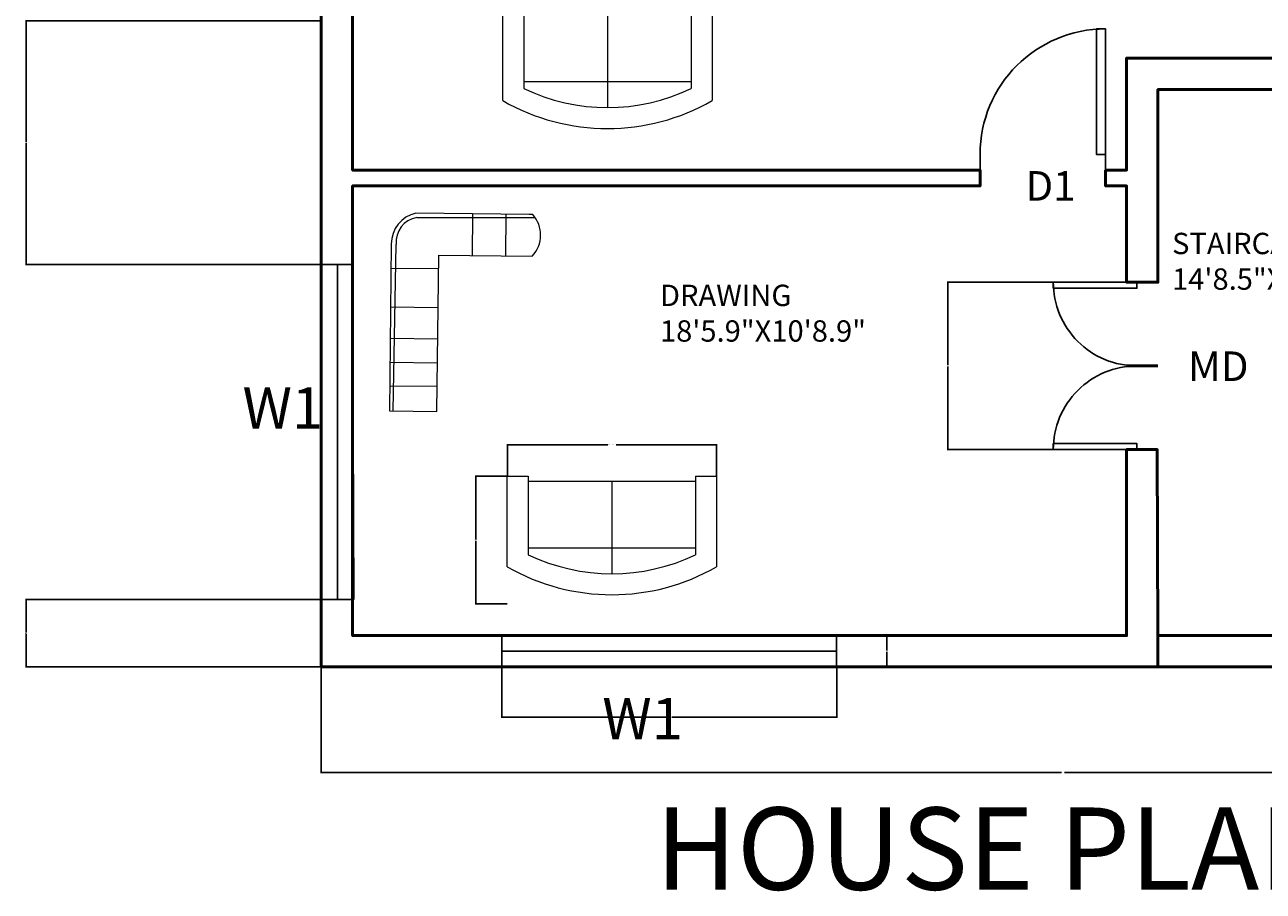
# Model space of a CAD drawing. Units: inches. Extents: x -45 to 1424, y 648 to 1662.
# Tile 1 of 8: x -45 to 310, y 648 to 896. Entities that reach past the tile are written whole.
import ezdxf

# ---------------------------------------------------------------- set-up
doc = ezdxf.new("R2010")
doc.units = ezdxf.units.IN
for name, color, linetype, lineweight in [('A-ANNO-DIMS', 2, 'Continuous', 18), ('A-ANNO-TEXT', 7, 'Continuous', 18), ('A-ANNO-TITL', 7, 'Continuous', 35), ('A-AREA-IDEN', 7, 'Continuous', 18), ('DOOR', 2, 'Continuous', 25), ('FURNITURE', 3, 'Continuous', 18), ('WALL', 4, 'Continuous', 50), ('WINDOW', 1, 'Continuous', 25)]:
    doc.layers.add(name, color=color, linetype=linetype, lineweight=lineweight)
doc.styles.get("Standard").update_dxf_attribs({"font": 'arial.ttf'})
doc.dimstyles.get("Standard").update_dxf_attribs({"dimtxt": 0.18, "dimasz": 0.18, "dimexe": 0.18, "dimexo": 0.0625, "dimgap": 0.09, "dimtad": 0, "dimtih": 1, "dimtoh": 1, "dimdec": 4, "dimzin": 0, "dimdsep": 46, "dimtxsty": 'Standard', "dimcen": 0.09, "dimadec": 0, "dimazin": 0, "dimtfac": 1, "dimtdec": 4, "dimtofl": 0, "dimtmove": 0, "dimatfit": 3, "dimfxl": 1, "dimtolj": 1, "dimtzin": 0, "dimarcsym": 0})

# ---------------------------------------------------------------- blocks, each defined once
blk = doc.blocks.new('*U3')
for p, q in [((0, 0), (0, -6)), ((24, 0), (24, -6))]:
    blk.add_line(p, q)
blk.add_lwpolyline([(0, 0), (0, 24), (1.75, 24), (1.75, 0)], close=True)
blk.add_arc((0, 0), 24, 0, 90)
blk = doc.blocks.new('*U6')
for p, q in [((0, 0), (0, 6)), ((24, 0), (24, 6))]:
    blk.add_line(p, q)
blk.add_lwpolyline([(0, 0), (0, -24), (1.75, -24), (1.75, 0)], close=True)
blk.add_arc((0, 0), 24, 270, 0)
blk = doc.blocks.new('Sofa - Roundback Loveseat 5 ft.')
for p, q in [((0, -32.44198), (0, -5.99998)), ((-24, -33.99998), (-24, -11.46958)), ((-23.9998, -13.38178), (23.99986, -13.38178)), ((24.00004, -33.99998), (24.00004, -11.46958)), ((-24, -32.44198), (24.00004, -32.44198))]:
    blk.add_line(p, q)
for points in [[(-24, -33.99998), (-30, -33.99998), (-30, -7.99998)], [(30.00004, -7.99998), (30.00004, -33.99998), (24.00004, -33.99998)]]:
    blk.add_lwpolyline(points)
for centre, radius, start, end in [((0, -60.24998), 60.24998, 60.13715, 119.8628), ((0, -61.38438), 55.38444, 64.32083, 115.6792)]:
    blk.add_arc(centre, radius, start, end)
blk = doc.blocks.new('WIN-W1-DRAWING-W')
for p, q in [((0, 96), (9, 96)), ((0, 0), (0, 96)), ((4.66, 0), (4.66, 96)), ((9, 96), (9.31, 0)), ((9.31, 0), (0, 0))]:
    blk.add_line(p, q)
blk = doc.blocks.new('WIN-W1-DRAWING-S')
for p, q in [((0, 9), (0, 0)), ((96, 9), (0, 9)), ((96, 0.07), (96, 9)), ((96, 4.53), (0, 4.53)), ((0, 0), (96, 0.07))]:
    blk.add_line(p, q)
blk = doc.blocks.new('FURN-CORNER-UNIT')
for p, q in [((40.07, 56.49), (7.6, 56.85)), ((7.84, 55.59), (41.8, 55.6)), ((23.84, 56.67), (23.71, 44.7)), ((33.42, 56.57), (33.29, 44.59)), ((41.09, 56.48), (40.07, 56.49)), ((0.52, 47.99), (0, 0.15)), ((1.05, 0.14), (1.97, 47.86)), ((13.64, 0), (14.13, 44.8)), ((14.13, 44.8), (40.96, 44.51)), ((14.09, 40.87), (0.45, 41.02)), ((13.96, 29.74), (0.33, 29.89)), ((13.86, 20.75), (0.23, 20.9)), ((13.79, 13.89), (0.15, 14.04)), ((13.72, 7.15), (0.08, 7.29)), ((0, 0.15), (13.64, 0))]:
    blk.add_line(p, q)
for centre, radius, start, end in [((9.61, 47.99), 9.08, 102.7689, 180), ((8.93, 48.68), 7, 98.9855, 186.697), ((34.55, 50.57), 8.82, 316.6036, 42.1383)]:
    blk.add_arc(centre, radius, start, end)
blk = doc.blocks.new('*D40')
at = {"layer": 'A-ANNO-DIMS', "color": 0, "lineweight": -2, "transparency": 16777216}
for p, q in [((93.37, 766.78), (93.37, 775.89)), ((93.55, 775.71), (122.14, 775.71)), ((153.19, 775.71), (124.59, 775.71)), ((153.37, 766.78), (153.37, 775.89))]:
    blk.add_line(p, q, dxfattribs=at)
at = {"layer": 'A-ANNO-DIMS', "color": 0, "transparency": 16777216}
for points in [[(93.55, 775.74), (93.55, 775.68), (93.37, 775.71)], [(153.19, 775.74), (153.19, 775.68), (153.37, 775.71)]]:
    blk.add_solid(points, dxfattribs=at)
at = {"layer": 'Defpoints', "color": 0, "transparency": 16777216}
for p in [(93.37, 775.71), (93.37, 766.71), (153.37, 766.71)]:
    blk.add_point(p, dxfattribs=at)
at = {"layer": 'A-ANNO-DIMS', "color": 0, "transparency": 16777216, "insert": (123.37, 775.71), "char_height": 0.18, "attachment_point": 5}
blk.add_mtext('\\A1;LOVESEAT 60 TYP.', dxfattribs=at)
blk = doc.blocks.new('*D41')
at = {"layer": 'A-ANNO-DIMS', "color": 0, "lineweight": -2, "transparency": 16777216}
for p, q in [((93.3, 766.71), (84.19, 766.71)), ((84.37, 766.53), (84.37, 748.56)), ((84.37, 730.23), (84.37, 748.2)), ((93.3, 730.05), (84.19, 730.05))]:
    blk.add_line(p, q, dxfattribs=at)
at = {"layer": 'A-ANNO-DIMS', "color": 0, "transparency": 16777216}
for points in [[(84.34, 766.53), (84.4, 766.53), (84.37, 766.71)], [(84.34, 730.23), (84.4, 730.23), (84.37, 730.05)]]:
    blk.add_solid(points, dxfattribs=at)
at = {"layer": 'Defpoints', "color": 0, "transparency": 16777216}
for p in [(93.37, 766.71), (84.37, 730.05), (93.37, 730.05)]:
    blk.add_point(p, dxfattribs=at)
at = {"layer": 'A-ANNO-DIMS', "color": 0, "transparency": 16777216, "insert": (84.37, 748.38), "char_height": 0.18, "attachment_point": 5}
blk.add_mtext('\\A1;37 TYP.', dxfattribs=at)
blk = doc.blocks.new('*D64')
at = {"layer": 'A-ANNO-DIMS', "color": 0, "lineweight": -2, "transparency": 16777216}
for p, q in [((91.8, 711.94), (91.8, 697.42)), ((187.8, 711.94), (187.8, 697.42)), ((91.98, 697.6), (139.04, 697.6)), ((187.62, 697.6), (140.55, 697.6))]:
    blk.add_line(p, q, dxfattribs=at)
at = {"layer": 'A-ANNO-DIMS', "color": 0, "transparency": 16777216}
for points in [[(91.98, 697.63), (91.98, 697.57), (91.8, 697.6)], [(187.62, 697.63), (187.62, 697.57), (187.8, 697.6)]]:
    blk.add_solid(points, dxfattribs=at)
at = {"layer": 'Defpoints', "color": 0, "transparency": 16777216}
for p in [(91.8, 712), (187.8, 712), (187.8, 697.6)]:
    blk.add_point(p, dxfattribs=at)
at = {"layer": 'A-ANNO-DIMS', "color": 0, "transparency": 16777216, "insert": (139.8, 697.6), "char_height": 0.18, "attachment_point": 5}
blk.add_mtext('\\A1;W1 96 TYP.', dxfattribs=at)
blk = doc.blocks.new('*D65')
at = {"layer": 'A-ANNO-DIMS', "color": 0, "lineweight": -2, "transparency": 16777216}
for p, q in [((187.86, 721), (202.38, 721)), ((202.2, 720.82), (202.2, 716.68)), ((202.2, 712.18), (202.2, 716.32)), ((187.86, 712), (202.38, 712))]:
    blk.add_line(p, q, dxfattribs=at)
at = {"layer": 'A-ANNO-DIMS', "color": 0, "transparency": 16777216}
for points in [[(202.17, 720.82), (202.23, 720.82), (202.2, 721)], [(202.17, 712.18), (202.23, 712.18), (202.2, 712)]]:
    blk.add_solid(points, dxfattribs=at)
at = {"layer": 'Defpoints', "color": 0, "transparency": 16777216}
for p in [(187.8, 721), (202.2, 721), (187.8, 712)]:
    blk.add_point(p, dxfattribs=at)
at = {"layer": 'A-ANNO-DIMS', "color": 0, "transparency": 16777216, "insert": (202.2, 716.5), "char_height": 0.18, "attachment_point": 5}
blk.add_mtext('\\A1;9 TYP.', dxfattribs=at)
blk = doc.blocks.new('*D74')
at = {"layer": 'A-ANNO-DIMS', "color": 0, "lineweight": -2, "transparency": 16777216}
for p, q in [((40, 711.94), (40, 681.57)), ((465.4, 711.94), (465.4, 681.57)), ((40.18, 681.75), (252.3, 681.75)), ((465.22, 681.75), (253.1, 681.75))]:
    blk.add_line(p, q, dxfattribs=at)
at = {"layer": 'A-ANNO-DIMS', "color": 0, "transparency": 16777216}
for points in [[(40.18, 681.78), (40.18, 681.72), (40, 681.75)], [(465.22, 681.78), (465.22, 681.72), (465.4, 681.75)]]:
    blk.add_solid(points, dxfattribs=at)
at = {"layer": 'Defpoints', "color": 0, "transparency": 16777216}
for p in [(40, 712), (465.4, 712), (465.4, 681.75)]:
    blk.add_point(p, dxfattribs=at)
at = {"layer": 'A-ANNO-DIMS', "color": 0, "transparency": 16777216, "insert": (252.7, 681.75), "char_height": 0.18, "attachment_point": 5}
blk.add_mtext('\\A1;425.4', dxfattribs=at)
blk = doc.blocks.new('*D79')
at = {"layer": 'A-ANNO-DIMS', "color": 0, "lineweight": -2, "transparency": 16777216}
for p, q in [((249.84, 822.29), (219.47, 822.29)), ((219.65, 822.11), (219.65, 798.47)), ((219.65, 774.47), (219.65, 798.11)), ((249.84, 774.29), (219.47, 774.29))]:
    blk.add_line(p, q, dxfattribs=at)
at = {"layer": 'A-ANNO-DIMS', "color": 0, "transparency": 16777216}
for points in [[(219.62, 822.11), (219.68, 822.11), (219.65, 822.29)], [(219.62, 774.47), (219.68, 774.47), (219.65, 774.29)]]:
    blk.add_solid(points, dxfattribs=at)
at = {"layer": 'Defpoints', "color": 0, "transparency": 16777216}
for p in [(219.65, 822.29), (249.9, 822.29), (249.9, 774.29)]:
    blk.add_point(p, dxfattribs=at)
at = {"layer": 'A-ANNO-DIMS', "color": 0, "transparency": 16777216, "insert": (219.65, 798.29), "char_height": 0.18, "attachment_point": 5}
blk.add_mtext('\\A1;48', dxfattribs=at)
blk = doc.blocks.new('*D87')
at = {"layer": 'A-ANNO-DIMS', "color": 0, "lineweight": -2, "transparency": 16777216}
for p, q in [((39.94, 731.33), (-44.82, 731.33)), ((-44.64, 731.15), (-44.64, 721.85)), ((-44.64, 712.18), (-44.64, 721.48)), ((39.94, 712), (-44.82, 712))]:
    blk.add_line(p, q, dxfattribs=at)
at = {"layer": 'A-ANNO-DIMS', "color": 0, "transparency": 16777216}
for points in [[(-44.67, 731.15), (-44.61, 731.15), (-44.64, 731.33)], [(-44.67, 712.18), (-44.61, 712.18), (-44.64, 712)]]:
    blk.add_solid(points, dxfattribs=at)
at = {"layer": 'Defpoints', "color": 0, "transparency": 16777216}
for p in [(-44.64, 731.33), (40, 731.33), (40, 712)]:
    blk.add_point(p, dxfattribs=at)
at = {"layer": 'A-ANNO-DIMS', "color": 0, "transparency": 16777216, "insert": (-44.64, 721.67), "char_height": 0.18, "attachment_point": 5}
blk.add_mtext('\\A1;19.33', dxfattribs=at)
blk = doc.blocks.new('*D88')
at = {"layer": 'A-ANNO-DIMS', "color": 0, "lineweight": -2, "transparency": 16777216}
for p, q in [((39.94, 897.23), (-44.82, 897.23)), ((-44.64, 897.05), (-44.64, 862.46)), ((-44.64, 827.51), (-44.64, 862.1)), ((39.94, 827.33), (-44.82, 827.33))]:
    blk.add_line(p, q, dxfattribs=at)
at = {"layer": 'A-ANNO-DIMS', "color": 0, "transparency": 16777216}
for points in [[(-44.67, 897.05), (-44.61, 897.05), (-44.64, 897.23)], [(-44.67, 827.51), (-44.61, 827.51), (-44.64, 827.33)]]:
    blk.add_solid(points, dxfattribs=at)
at = {"layer": 'Defpoints', "color": 0, "transparency": 16777216}
for p in [(-44.64, 897.23), (40, 897.23), (40, 827.33)]:
    blk.add_point(p, dxfattribs=at)
at = {"layer": 'A-ANNO-DIMS', "color": 0, "transparency": 16777216, "insert": (-44.64, 862.28), "char_height": 0.18, "attachment_point": 5}
blk.add_mtext('\\A1;69.9', dxfattribs=at)

msp = doc.modelspace()

# ---------------------------------------------------------------- linework, layer by layer
at = {"layer": 'WALL'}
msp.add_line((279.9, 798.2916), (270.9, 798.2916), dxfattribs=at)
msp.add_lwpolyline([(465.4, 1180), (465.4, 712), (40, 712), (40, 1180)], close=True, dxfattribs=at)
for points in [[(279.9, 712), (279.9, 721), (279.7284, 774.2923), (270.9, 774.2923), (270.9, 721), (49, 721), (49, 849.9), (228.9004, 849.9), (228.9004, 854.4), (49, 854.4), (49, 1024), (144.0001, 1024)], [(370.3983, 886.5), (364.4, 886.5), (364.4, 892.4923), (359.9, 892.4923), (359.9, 886.5), (270.9, 886.5), (270.9, 854.4), (264.9004, 854.4)], [(279.9, 822.291), (279.9, 877.5), (279.9, 822.291), (270.9, 822.291), (270.9, 849.9), (264.9004, 849.9), (264.9004, 854.4)], [(279.9, 877.5), (456.4, 877.5), (456.4, 721), (279.9, 721)]]:
    msp.add_lwpolyline(points, dxfattribs=at)

# ---------------------------------------------------------------- block references
at = {"layer": 'DOOR', "xscale": -1.5, "yscale": 1.5, "zscale": 1.5}
msp.add_blockref('*U3', (264.9004, 858.9), dxfattribs=at)
at = {"layer": 'DOOR', "rotation": 270}
msp.add_blockref('*U6', (273.9, 822.2916), dxfattribs=at)
at = {"layer": 'DOOR', "xscale": -1, "rotation": 270}
msp.add_blockref('*U6', (273.9, 774.2916), dxfattribs=at)
at = {"layer": 'FURNITURE', "rotation": 180}
for p in [(122.0801, 866.3268), (123.366, 732.7133)]:
    msp.add_blockref('Sofa - Roundback Loveseat 5 ft.', p, dxfattribs=at)
at = {"layer": 'FURNITURE'}
msp.add_blockref('FURN-CORNER-UNIT', (59.554, 785.232), dxfattribs=at)
at = {"layer": 'WINDOW'}
for name, p in [('WIN-W1-DRAWING-W', (40, 731.331)), ('WIN-W1-DRAWING-S', (91.796, 712))]:
    msp.add_blockref(name, p, dxfattribs=at)

# ---------------------------------------------------------------- texts
at = {"layer": 'A-ANNO-TEXT', "attachment_point": 1}
for s, width, gutter_width, insert, char_height in [('D1', 8.475535, 42.3777, (241.9287, 854.1229), 8.47554), ('MD', 8.475535, 42.3777, (288.5439, 802.4339), 8.47554), ('W1', 18.68524, 59.1031, (17.4497, 792.1583), 11.82062), ('W1', 18.68524, 59.1031, (120.5987, 703.1192), 11.82062)]:
    msp.add_mtext_dynamic_manual_height_columns(s, width=width, gutter_width=gutter_width, heights=[0], dxfattribs=dict(at, insert=insert, char_height=char_height))
at = {"layer": 'A-ANNO-TITL', "insert": (135.7629, 671.7231), "char_height": 23.5814, "attachment_point": 1}
msp.add_mtext('HOUSE PLAN', dxfattribs=at)
at = {"layer": 'A-AREA-IDEN', "char_height": 6.122202, "attachment_point": 1}
for s, insert in [('STAIRCASE\\P14\'8.5"X13\'0.5"', (283.9629, 836.4432)), ('DRAWING\\P18\'5.9"X10\'8.9"', (137.1322, 821.5647))]:
    msp.add_mtext(s, dxfattribs=dict(at, insert=insert))

# ---------------------------------------------------------------- dimensions: what is measured, and where the dimension line sits
at = {"layer": 'A-ANNO-DIMS'}
for base, p1, p2, override, picture, middle in [((-44.6411, 897.2341), (40, 827.3302), (40, 897.2341), {"dimdec": 1, "dimlfac": 1, "dimrnd": 0, "dimzin": 0, "dimdsep": 46, "dimlunit": 2}, '*D88', (-44.6411, 862.2822)), ((219.65, 822.2916), (249.9, 774.2916), (249.9, 822.2916), {"dimdec": 0, "dimlfac": 1, "dimrnd": 0, "dimzin": 0, "dimdsep": 46, "dimlunit": 2}, '*D79', (219.65, 798.2916)), ((-44.6411, 731.3307), (40, 712), (40, 731.3307), {"dimdec": 2, "dimlfac": 1, "dimrnd": 0, "dimzin": 0, "dimdsep": 46, "dimlunit": 2}, '*D87', (-44.6411, 721.6654))]:
    dim = msp.add_linear_dim(base=base, p1=p1, p2=p2, angle=90, dimstyle='Standard', override=override, dxfattribs=at)
    dim.commit()
    dim.dimension.update_dxf_attribs({"geometry": picture, "text_midpoint": middle})
for base, p1, p2, angle, text, picture, middle in [((93.3659, 775.7133), (153.366, 766.7133), (93.3659, 766.7133), 180, 'LOVESEAT <> TYP.', '*D40', (123.366, 775.7133)), ((84.3659, 730.0467), (93.3659, 766.7133), (93.3659, 730.0467), 270, '<> TYP.', '*D41', (84.3659, 748.38)), ((202.1961, 721), (187.7961, 712), (187.7961, 721), 90, '<> TYP.', '*D65', (202.1961, 716.5))]:
    dim = msp.add_linear_dim(base=base, p1=p1, p2=p2, angle=angle, text=text, dimstyle='Standard', override={"dimdec": 0, "dimlfac": 1, "dimrnd": 0, "dimzin": 0, "dimdsep": 46, "dimlunit": 2}, dxfattribs=at)
    dim.commit()
    dim.dimension.update_dxf_attribs({"geometry": picture, "text_midpoint": middle})
dim = msp.add_linear_dim(base=(465.4, 681.75), p1=(40, 712), p2=(465.4, 712), dimstyle='Standard', override={"dimdec": 1, "dimlfac": 1, "dimrnd": 0, "dimzin": 0, "dimdsep": 46, "dimlunit": 2}, dxfattribs=at)
dim.commit()
dim.dimension.update_dxf_attribs({"geometry": '*D74', "text_midpoint": (252.7, 681.75)})
dim = msp.add_linear_dim(base=(187.7961, 697.6), p1=(91.7961, 712), p2=(187.7961, 712), text='W1 <> TYP.', dimstyle='Standard', override={"dimdec": 0, "dimlfac": 1, "dimrnd": 0, "dimzin": 0, "dimdsep": 46, "dimlunit": 2}, dxfattribs=at)
dim.commit()
dim.dimension.update_dxf_attribs({"geometry": '*D64', "text_midpoint": (139.7961, 697.6)})

doc.saveas('drawing.dxf')
